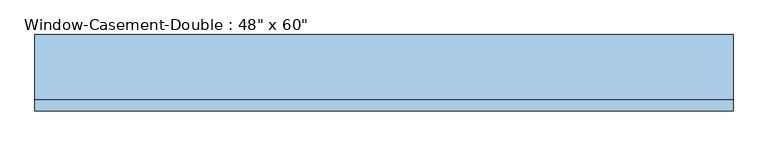
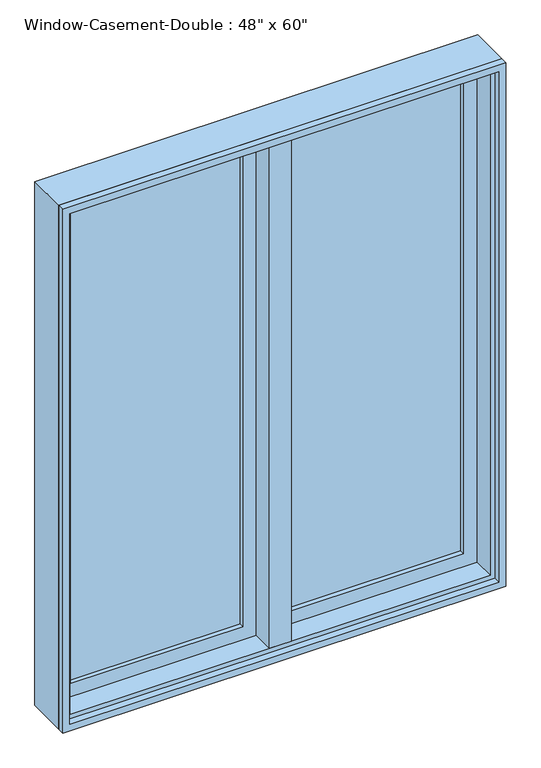
"""IFC4 building model written with IfcOpenShell, lengths in millimetres: window geometry."""

from ifc_helpers import new_model, si_unit, frame, origin, place, context, project, spatial, polyline, outline, extrude, faceted_brep, source, transform, mapped, element, save


def window_d9d3dda5(model_context):
    return source(origin(), model_context, "Body", "SolidModel", [
        faceted_brep([(9.525, 76.2, 2425.7), (-9.525, 76.2, 2425.7), (-9.525, 25.4, 2425.7), (9.525, 25.4, 2425.7), (9.525, 76.2, 927.1), (9.525, 25.4, 927.1), (-9.525, 25.4, 927.1), (-9.525, 76.2, 927.1), (-9.525, 25.4, 946.15), (-9.525, 25.4, 2406.65), (-30.1625, 25.4, 946.15), (-30.1625, 25.4, 2406.65), (-30.1625, -38.1, 946.15), (-30.1625, -38.1, 2406.65), (30.1625, -38.1, 946.15), (30.1625, -38.1, 2406.65), (30.1625, 25.4, 946.15), (30.1625, 25.4, 2406.65), (9.525, 25.4, 946.15), (9.525, 25.4, 2406.65)], [[[0, 1, 2, 3]], [[4, 5, 6, 7]], [[1, 0, 4, 7]], [[2, 1, 7, 6, 8, 9]], [[9, 8, 10, 11]], [[11, 10, 12, 13]], [[13, 12, 14, 15]], [[15, 14, 16, 17]], [[17, 16, 18, 19]], [[0, 3, 19, 18, 5, 4]], [[18, 8, 6, 5]], [[9, 19, 3, 2]], [[8, 18, 16, 14, 12, 10]], [[19, 9, 11, 13, 15, 17]]]),
        extrude(outline(polyline([(-66.675, 57.15), (-66.675, 50.8), (-539.75, 50.8), (-539.75, 57.15), (-66.675, 57.15)])), frame((0.0, 0.0, 984.25), z_axis=(0.0, 0.0, 1.0), x_axis=(1.0, 0.0, 0.0)), (0.0, 0.0, 1.0), 1384.3),
        extrude(outline(polyline([(-539.75, 38.1), (-539.75, 44.45), (-66.675, 44.45), (-66.675, 38.1), (-539.75, 38.1)])), frame((0.0, 0.0, 984.25), z_axis=(0.0, 0.0, 1.0), x_axis=(1.0, 0.0, 0.0)), (0.0, 0.0, 1.0), 1384.3),
        extrude(outline(polyline([(539.75, 57.15), (539.75, 50.8), (66.675, 50.8), (66.675, 57.15), (539.75, 57.15)])), frame((0.0, 0.0, 984.25), z_axis=(0.0, 0.0, 1.0), x_axis=(1.0, 0.0, 0.0)), (0.0, 0.0, 1.0), 1384.3),
        extrude(outline(polyline([(66.675, 38.1), (66.675, 44.45), (539.75, 44.45), (539.75, 38.1), (66.675, 38.1)])), frame((0.0, 0.0, 984.25), z_axis=(0.0, 0.0, 1.0), x_axis=(1.0, 0.0, 0.0)), (0.0, 0.0, 1.0), 1384.3),
        extrude(outline(polyline([(2425.7, -596.9), (927.1, -596.9), (927.1, -9.525), (2425.7, -9.525), (2425.7, -596.9)]), holes=[polyline([(2368.55, -66.675), (984.25, -66.675), (984.25, -539.75), (2368.55, -539.75), (2368.55, -66.675)])]), frame((0.0, 25.4, 0.0), z_axis=(0.0, 1.0, 0.0), x_axis=(0.0, 0.0, 1.0)), (0.0, 0.0, 1.0), 44.45),
        extrude(outline(polyline([(927.1, 596.9), (2425.7, 596.9), (2425.7, 9.525), (927.1, 9.525), (927.1, 596.9)]), holes=[polyline([(984.25, 66.675), (2368.55, 66.675), (2368.55, 539.75), (984.25, 539.75), (984.25, 66.675)])]), frame((0.0, 25.4, 0.0), z_axis=(0.0, 1.0, 0.0), x_axis=(0.0, 0.0, 1.0)), (0.0, 0.0, 1.0), 44.45),
        extrude(outline(polyline([(2438.4, -609.6), (914.4, -609.6), (914.4, 609.6), (2438.4, 609.6), (2438.4, -609.6)]), holes=[polyline([(2419.35, 590.55), (933.45, 590.55), (933.45, -590.55), (2419.35, -590.55), (2419.35, 590.55)])]), frame((0.0, -57.15, 0.0), z_axis=(0.0, 1.0, 0.0), x_axis=(0.0, 0.0, 1.0)), (0.0, 0.0, 1.0), 19.05),
        faceted_brep([(577.85, 25.4, 2406.65), (577.85, -38.1, 2406.65), (-577.85, -38.1, 2406.65), (-577.85, 25.4, 2406.65), (596.9, 76.2, 2425.7), (596.9, 25.4, 2425.7), (-596.9, 25.4, 2425.7), (-596.9, 76.2, 2425.7), (609.6, -38.1, 2438.4), (609.6, 76.2, 2438.4), (-609.6, 76.2, 2438.4), (-609.6, -38.1, 2438.4), (-577.85, -38.1, 946.15), (-577.85, 25.4, 946.15), (-596.9, 25.4, 927.1), (-596.9, 76.2, 927.1), (-609.6, 76.2, 914.4), (-609.6, -38.1, 914.4), (577.85, -38.1, 946.15), (577.85, 25.4, 946.15), (596.9, 25.4, 927.1), (596.9, 76.2, 927.1), (609.6, 76.2, 914.4), (609.6, -38.1, 914.4)], [[[0, 1, 2, 3]], [[4, 5, 6, 7]], [[8, 9, 10, 11]], [[3, 2, 12, 13]], [[7, 6, 14, 15]], [[11, 10, 16, 17]], [[13, 12, 18, 19]], [[15, 14, 20, 21]], [[17, 16, 22, 23]], [[11, 17, 23, 8], [1, 18, 12, 2]], [[19, 18, 1, 0]], [[5, 20, 14, 6], [3, 13, 19, 0]], [[21, 20, 5, 4]], [[23, 22, 9, 8]], [[9, 22, 16, 10], [7, 15, 21, 4]]]),
    ])


if __name__ == "__main__":
    model = new_model("IFC4")
    model_context = context("Model", 3, world=origin())
    ifc_project = project(units=[si_unit("LENGTHUNIT", "METRE", prefix="MILLI")], contexts=[model_context])
    site = spatial("IfcSite", under=ifc_project)
    building = spatial("IfcBuilding", under=site)
    placement = place(None, origin())
    window_shape = window_d9d3dda5(model_context)
    element("IfcWindow", 1, ObjectType="Window-Casement-Double : 48\" x 60\"", at=placement, inside=building, context=model_context, shape_type="MappedRepresentation", body=[
        mapped(window_shape, transform((0.0, 0.0, 0.0), x_axis=(1.0, 0.0, 0.0), y_axis=(0.0, 1.0, 0.0), z_axis=(0.0, 0.0, 1.0))),
    ])
    save(model, "model.ifc")

# Revit data of these elements
# Type "Window-Casement-Double : 48\" x 60\""
#   Type Mark = "17"
#   Fire Rating = "0.5h"
#   Assembly Code = "B2020100"
#   Analytic Construction = "Double glazing - domestic"
#   Frame Extension [instance default] = 0' - 0 1/4"
#   Window Inset [instance default] = 0' - 0"
#   Wall Thickness [instance default] = 0' - 6"
#   Interior Wall Closure [instance default] = 0' - 2 1/4"
#   Half Width = 2' - 0"
#   Visual Light Transmittance = 0.81
#   Thermal Resistance (R) = 1.8146 (h·ft²·°F)/BTU
#   Solar Heat Gain Coefficient = 0.76
#   Rough Width = 4' - 0 1/2"
#   Rough Height = 5' - 0 1/2"
#   Height = 5' - 0"
#   Heat Transfer Coefficient (U) = 0.5511 BTU/(h·ft²·°F)
#   Exterior Wall Closure [instance default] = 0' - 1 1/4"
#   Extension Jamb [instance default] = 0' - 2 1/4"
#   Default Sill Height = 3' - 0"
#   Width = 4' - 0"
#   Define Thermal Properties by = 0
#   Muntin Visibility = yes
#   Interior Trim Visibility [instance default] = yes
#   Exterior Trim Visibility [instance default] = yes
#   Extension Jamb Visibility [instance default] = yes
#   Interior Trim Material = Wood - Stained
#   Muntin Pattern = Muntin Pattern_2x2 : Muntin Pattern_2x2
#   Interior Trim = Trim-Window-Interior-Flat : Picture Frame
#   Interior Frame Material = Wood - Stained
#   Glass Panel Material = Glass
#   Exterior Trim Material = Clad - White
#   Exterior Trim = Trim-Window-Exterior-Flat : with Sill
#   Exterior Frame Material = Clad - White
#   Wall Closure = (empty or 0)
# Element 1 (IfcWindow, "Window-Casement-Double : 48\" x 60\"")
#   Wall Thickness = 0' - 4 1/2"
#   Extension Jamb = 0' - 0 3/4"
#   Materials on its faces: "Wood - Stained", "Glass", "Clad - White"
# Materials
#   "Wood - Stained": class "Wood", colour RGB 224 178 126, transparency 0, Cost = 0
#   "Glass": class "Glass", colour RGB 0 128 192, transparency 0.75, Description = "Soda Lime Glass", Cost = 0
#   "Clad - White": class "Wood", colour RGB 242 242 238, transparency 0, Cost = 0
